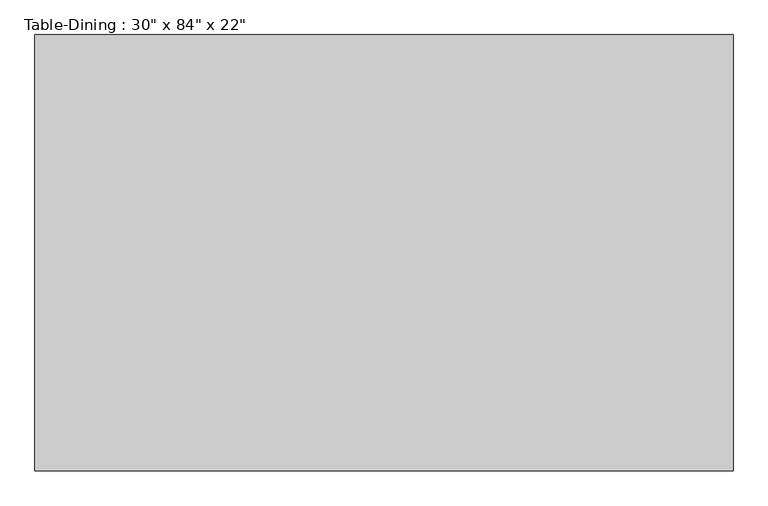
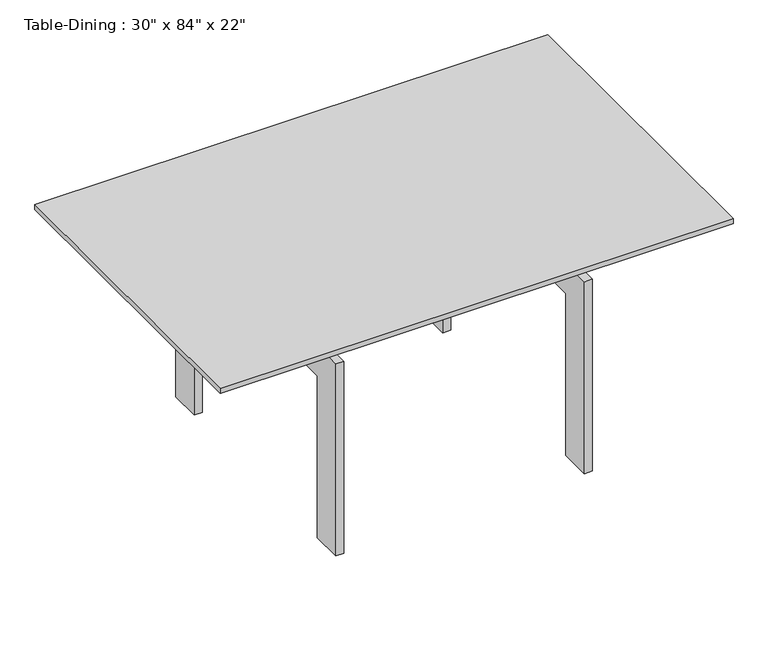
"""IFC4 building model written with IfcOpenShell, lengths in millimetres: furniture geometry."""

from ifc_helpers import new_model, si_unit, frame, origin, place, context, project, spatial, polyline, outline, extrude, source, transform, mapped, element, save


def furniture_e3bc833e(model_context):
    return source(origin(), model_context, "Body", "SweptSolid", [
        extrude(outline(polyline([(526.2657667, 297.7823857), (526.2657667, 272.3823857), (-489.7342333, 272.3823857), (-489.7342333, 297.7823857), (526.2657667, 297.7823857)])), frame((0.0, 0.0, 482.6), z_axis=(0.0, 0.0, 1.0), x_axis=(1.0, 0.0, 0.0)), (0.0, 0.0, 1.0), 63.5),
        extrude(outline(polyline([(526.2657667, -82.5889222), (526.2657667, -107.9889222), (-489.7342333, -107.9889222), (-489.7342333, -82.5889222), (526.2657667, -82.5889222)])), frame((0.0, 0.0, 482.6), z_axis=(0.0, 0.0, 1.0), x_axis=(1.0, 0.0, 0.0)), (0.0, 0.0, 1.0), 63.5),
        extrude(outline(polyline([(425.4110778, 0.0), (349.2110778, 0.0), (349.2110778, 406.4), (-158.7889222, 406.4), (-158.7889222, 0.0), (-234.9889222, 0.0), (-234.9889222, 482.6), (425.4110778, 482.6), (425.4110778, 0.0)])), frame((304.0157667, 0.0, 0.0), z_axis=(1.0, 0.0, 0.0), x_axis=(0.0, 1.0, 0.0)), (0.0, 0.0, 1.0), 19.05),
        extrude(outline(polyline([(425.4110778, 482.6), (425.4110778, 0.0), (349.2110778, 0.0), (349.2110778, 406.4), (-158.7889222, 406.4), (-158.7889222, 0.0), (-234.9889222, 0.0), (-234.9889222, 482.6), (425.4110778, 482.6)])), frame((-286.5342333, 0.0, 0.0), z_axis=(1.0, 0.0, 0.0), x_axis=(0.0, 1.0, 0.0)), (0.0, 0.0, 1.0), 19.05),
        extrude(outline(polyline([(627.8657667, 476.2110778), (627.8657667, -285.7889222), (-591.3342333, -285.7889222), (-591.3342333, 476.2110778), (627.8657667, 476.2110778)])), frame((0.0, 0.0, 546.1), z_axis=(0.0, 0.0, 1.0), x_axis=(1.0, 0.0, 0.0)), (0.0, 0.0, 1.0), 12.7),
    ])


if __name__ == "__main__":
    model = new_model("IFC4")
    model_context = context("Model", 3, world=origin())
    ifc_project = project(units=[si_unit("LENGTHUNIT", "METRE", prefix="MILLI")], contexts=[model_context])
    site = spatial("IfcSite", under=ifc_project)
    building = spatial("IfcBuilding", under=site)
    placement = place(None, origin())
    furniture_shape = furniture_e3bc833e(model_context)
    element("IfcFurniture", 1, ObjectType="Table-Dining : 30\" x 84\" x 22\"", at=placement, inside=building, context=model_context, shape_type="MappedRepresentation", body=[
        mapped(furniture_shape, transform((0.0, 0.0, 0.0), x_axis=(1.0, 0.0, 0.0), y_axis=(0.0, 1.0, 0.0), z_axis=(0.0, 0.0, 1.0))),
    ])
    save(model, "model.ifc")

# Revit data of these elements
# Type "Table-Dining : 30\" x 84\" x 22\""
#   Assembly Code = "E2020200"
#   Height = 1' - 10"
#   Length = 4' - 0"
#   Width = 2' - 6"
#   Base Material = Steel, Chrome Plated
#   Top Material = Glass - Clear, Grey
#   Default Elevation = 0
# Element 1 (IfcFurniture, "Table-Dining : 30\" x 84\" x 22\"")
#   Materials on its faces: "Steel, Chrome Plated", "Glass - Clear, Grey"
# Materials
#   "Steel, Chrome Plated": class "Metal", colour RGB 17 17 17, transparency 0, Description = "Chromiuim plated steel", Cost = 0
#   "Glass - Clear, Grey": class "Glass", colour RGB 252 255 255, transparency 0.64
